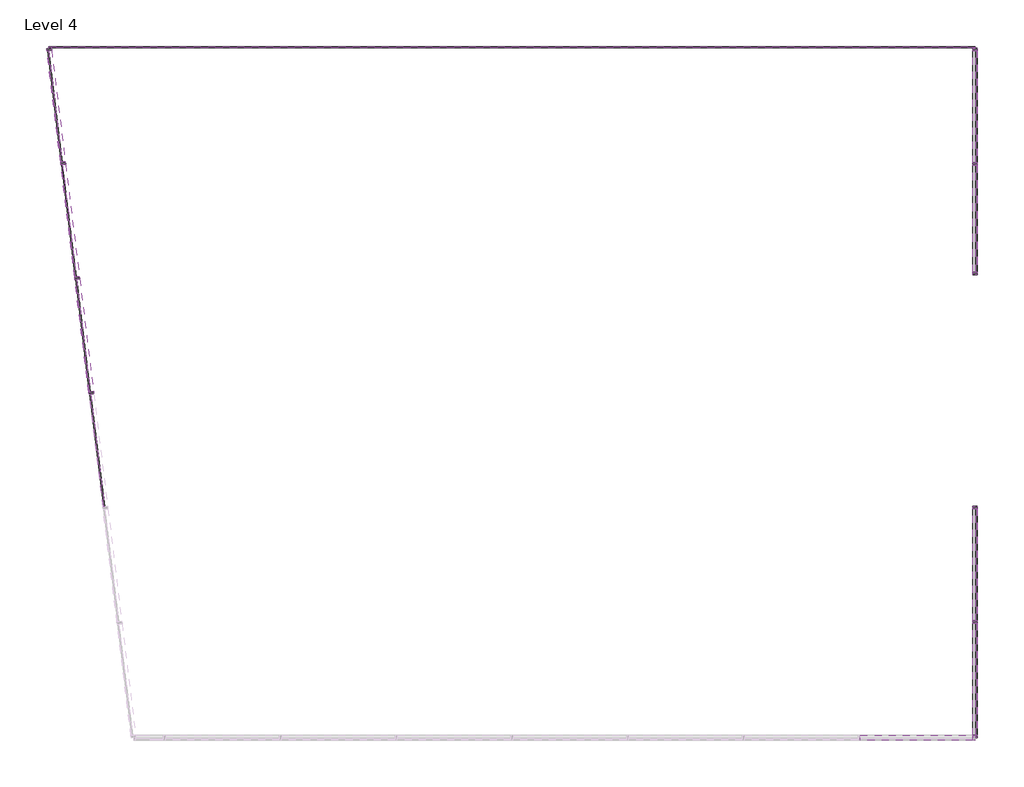
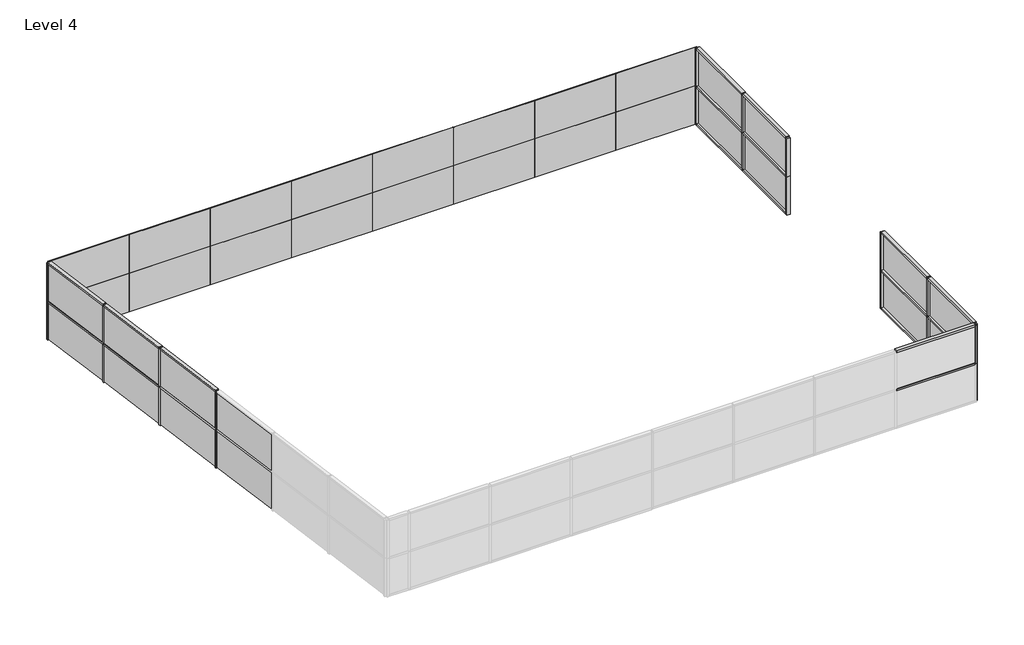
# One storey, part 2 of 2: 41 members, 32 plates.
"""IFC4 building model written with IfcOpenShell, lengths in millimetres."""

from ifc_helpers import new_model, si_unit, origin, place, context, project, spatial, transform, mapped, element, save
from components import member_71c27fd2, member_19d0a4ec, member_8cef0660, member_82905deb, member_4491d118, member_1b94d493, member_46bdb8c2, system_panel_glazed_1e57f9bb, system_panel_glazed_37f15d2e, system_panel_glazed_e46d4b42, system_panel_glazed_2a6c68b7, system_panel_glazed_7fb1fc2b, system_panel_glazed_d483336f

model = new_model("IFC4")

# Units and contexts
model_context = context("Model", 3, world=origin())
ifc_project = project(units=[si_unit("LENGTHUNIT", "METRE", prefix="MILLI")], contexts=[model_context])

# Site, building, storey
site = spatial("IfcSite", under=ifc_project)
building = spatial("IfcBuilding", under=site)
storey = spatial("IfcBuildingStorey", under=building, Name="Level 4", Elevation=9144.0)

# Members
placement = place(None, origin())
member_shape = member_71c27fd2(model_context)
element("IfcMember", 1, ObjectType="Rectangular Mullion : 2.5\" x 5\" rectangular", at=placement, inside=storey, context=model_context, shape_type="MappedRepresentation", body=[
    mapped(member_shape, transform((13902.5156363, -6915.6363705, 9144.0), x_axis=(0.0, 0.0, -1.0), y_axis=(1.0, 0.0, 0.0), z_axis=(0.0, -1.0, 0.0))),
])
element("IfcMember", 2, ObjectType="Rectangular Mullion : 2.5\" x 5\" rectangular", at=placement, inside=storey, context=model_context, shape_type="MappedRepresentation", body=[
    mapped(member_shape, transform((13902.5156363, -3899.3863708, 9144.0), x_axis=(0.0, 0.0, -1.0), y_axis=(1.0, 0.0, 0.0), z_axis=(0.0, -1.0, 0.0))),
])
element("IfcMember", 3, ObjectType="Rectangular Mullion : 2.5\" x 5\" rectangular", at=placement, inside=storey, context=model_context, shape_type="MappedRepresentation", body=[
    mapped(member_shape, transform((13902.5156363, 8156.2976505, 9144.0), x_axis=(0.0, 0.0, -1.0), y_axis=(1.0, 0.0, 0.0), z_axis=(0.0, -1.0, 0.0))),
])
member_2_shape = member_19d0a4ec(model_context)
element("IfcMember", 4, ObjectType="Rectangular Mullion : 2.5\" x 5\" rectangular", at=placement, inside=storey, context=model_context, shape_type="MappedRepresentation", body=[
    mapped(member_2_shape, transform((13839.0156363, -6979.1363705, 10668.0), x_axis=(0.0, 0.0, 1.0), y_axis=(0.0, -1.0, 0.0), z_axis=(1.0, 0.0, 0.0))),
])
element("IfcMember", 5, ObjectType="Rectangular Mullion : 2.5\" x 5\" rectangular", at=placement, inside=storey, context=model_context, shape_type="MappedRepresentation", body=[
    mapped(member_2_shape, transform((13839.0156363, -6979.1363705, 12192.0), x_axis=(0.0, 0.0, 1.0), y_axis=(0.0, -1.0, 0.0), z_axis=(1.0, 0.0, 0.0))),
])
element("IfcMember", 6, ObjectType="Rectangular Mullion : 2.5\" x 5\" rectangular", at=placement, inside=storey, context=model_context, shape_type="MappedRepresentation", body=[
    mapped(member_2_shape, transform((-10113.8959567, 8178.7803212, 10668.0), x_axis=(0.0, 0.0, 1.0), y_axis=(-0.9925461516413222, -0.12186934340514609, 0.0), z_axis=(0.12186934340514609, -0.9925461516413222, 0.0))),
])
element("IfcMember", 7, ObjectType="Rectangular Mullion : 2.5\" x 5\" rectangular", at=placement, inside=storey, context=model_context, shape_type="MappedRepresentation", body=[
    mapped(member_2_shape, transform((-10113.8959567, 8178.7803212, 12192.0), x_axis=(0.0, 0.0, 1.0), y_axis=(-0.9925461516413222, -0.12186934340514617, 0.0), z_axis=(0.12186934340514617, -0.9925461516413222, 0.0))),
])
element("IfcMember", 8, ObjectType="Rectangular Mullion : 2.5\" x 5\" rectangular", at=placement, inside=storey, context=model_context, shape_type="MappedRepresentation", body=[
    mapped(member_2_shape, transform((13902.5156363, -946.6363705, 10668.0), x_axis=(0.0, 0.0, 1.0), y_axis=(1.0, 0.0, 0.0), z_axis=(0.0, 1.0, 0.0))),
])
element("IfcMember", 9, ObjectType="Rectangular Mullion : 2.5\" x 5\" rectangular", at=placement, inside=storey, context=model_context, shape_type="MappedRepresentation", body=[
    mapped(member_2_shape, transform((13902.5156363, -3962.8863708, 10668.0), x_axis=(0.0, 0.0, 1.0), y_axis=(1.0, 0.0, 0.0), z_axis=(0.0, 1.0, 0.0))),
])
element("IfcMember", 10, ObjectType="Rectangular Mullion : 2.5\" x 5\" rectangular", at=placement, inside=storey, context=model_context, shape_type="MappedRepresentation", body=[
    mapped(member_2_shape, transform((13902.5156363, -946.6363705, 12192.0), x_axis=(0.0, 0.0, 1.0), y_axis=(1.0, 0.0, 0.0), z_axis=(0.0, 1.0, 0.0))),
])
element("IfcMember", 11, ObjectType="Rectangular Mullion : 2.5\" x 5\" rectangular", at=placement, inside=storey, context=model_context, shape_type="MappedRepresentation", body=[
    mapped(member_2_shape, transform((13902.5156363, -3962.8863708, 12192.0), x_axis=(0.0, 0.0, 1.0), y_axis=(1.0, 0.0, 0.0), z_axis=(0.0, 1.0, 0.0))),
])
element("IfcMember", 12, ObjectType="Rectangular Mullion : 2.5\" x 5\" rectangular", at=placement, inside=storey, context=model_context, shape_type="MappedRepresentation", body=[
    mapped(member_2_shape, transform((13902.5156363, 11109.0476508, 10668.0), x_axis=(0.0, 0.0, 1.0), y_axis=(1.0, 0.0, 0.0), z_axis=(0.0, 1.0, 0.0))),
])
element("IfcMember", 13, ObjectType="Rectangular Mullion : 2.5\" x 5\" rectangular", at=placement, inside=storey, context=model_context, shape_type="MappedRepresentation", body=[
    mapped(member_2_shape, transform((13902.5156363, 11109.0476508, 12192.0), x_axis=(0.0, 0.0, 1.0), y_axis=(1.0, 0.0, 0.0), z_axis=(0.0, 1.0, 0.0))),
])
member_3_shape = member_8cef0660(model_context)
element("IfcMember", 14, ObjectType="Rectangular Mullion : 2.5\" x 5\" rectangular", at=placement, inside=storey, context=model_context, shape_type="MappedRepresentation", body=[
    mapped(member_3_shape, transform((-9370.9804393, 2128.2189808, 10668.0), x_axis=(0.0, 0.0, 1.0), y_axis=(-0.9925461516413223, -0.12186934340514563, 0.0), z_axis=(0.12186934340514562, -0.9925461516413222, 0.0))),
])
element("IfcMember", 15, ObjectType="Rectangular Mullion : 2.5\" x 5\" rectangular", at=placement, inside=storey, context=model_context, shape_type="MappedRepresentation", body=[
    mapped(member_3_shape, transform((-9742.438198, 5153.499651, 10668.0), x_axis=(0.0, 0.0, 1.0), y_axis=(-0.9925461516413222, -0.12186934340514602, 0.0), z_axis=(0.12186934340514602, -0.9925461516413222, 0.0))),
])
element("IfcMember", 16, ObjectType="Rectangular Mullion : 2.5\" x 5\" rectangular", at=placement, inside=storey, context=model_context, shape_type="MappedRepresentation", body=[
    mapped(member_3_shape, transform((-9370.9804393, 2128.2189808, 12192.0), x_axis=(0.0, 0.0, 1.0), y_axis=(-0.9925461516413222, -0.12186934340514596, 0.0), z_axis=(0.12186934340514596, -0.9925461516413222, 0.0))),
])
element("IfcMember", 17, ObjectType="Rectangular Mullion : 2.5\" x 5\" rectangular", at=placement, inside=storey, context=model_context, shape_type="MappedRepresentation", body=[
    mapped(member_3_shape, transform((-9742.438198, 5153.499651, 12192.0), x_axis=(0.0, 0.0, 1.0), y_axis=(-0.9925461516413222, -0.12186934340514566, 0.0), z_axis=(0.12186934340514566, -0.9925461516413222, 0.0))),
])
member_4_shape = member_82905deb(model_context)
element("IfcMember", 18, ObjectType="Rectangular Mullion : 2.5\" x 5\" rectangular", at=placement, inside=storey, context=model_context, shape_type="MappedRepresentation", body=[
    mapped(member_4_shape, transform((13902.5156363, -3931.1363708, 10668.0), x_axis=(0.0, -1.0, 0.0), y_axis=(1.0, 0.0, 0.0), z_axis=(0.0, 0.0, 1.0))),
])
element("IfcMember", 19, ObjectType="Rectangular Mullion : 2.5\" x 5\" rectangular", at=placement, inside=storey, context=model_context, shape_type="MappedRepresentation", body=[
    mapped(member_4_shape, transform((13902.5156363, 8124.5476505, 10668.0), x_axis=(0.0, -1.0, 0.0), y_axis=(1.0, 0.0, 0.0), z_axis=(0.0, 0.0, 1.0))),
])
element("IfcMember", 20, ObjectType="Rectangular Mullion : 2.5\" x 5\" rectangular", at=placement, inside=storey, context=model_context, shape_type="MappedRepresentation", body=[
    mapped(member_4_shape, transform((-9367.1110876, 2096.7056405, 10668.0), x_axis=(-0.1218693434051459, 0.9925461516413222, 0.0), y_axis=(-0.9925461516413222, -0.1218693434051459, 0.0), z_axis=(0.0, 0.0, 1.0))),
])
element("IfcMember", 21, ObjectType="Rectangular Mullion : 2.5\" x 5\" rectangular", at=placement, inside=storey, context=model_context, shape_type="MappedRepresentation", body=[
    mapped(member_4_shape, transform((-9367.1110876, 2096.7056405, 12192.0), x_axis=(-0.1218693434051459, 0.9925461516413222, 0.0), y_axis=(-0.9925461516413222, -0.1218693434051459, 0.0), z_axis=(0.0, 0.0, 1.0))),
])
element("IfcMember", 22, ObjectType="Rectangular Mullion : 2.5\" x 5\" rectangular", at=placement, inside=storey, context=model_context, shape_type="MappedRepresentation", body=[
    mapped(member_4_shape, transform((-9738.5688463, 5121.9863107, 10668.0), x_axis=(-0.1218693434051459, 0.9925461516413222, 0.0), y_axis=(-0.9925461516413222, -0.1218693434051459, 0.0), z_axis=(0.0, 0.0, 1.0))),
])
element("IfcMember", 23, ObjectType="Rectangular Mullion : 2.5\" x 5\" rectangular", at=placement, inside=storey, context=model_context, shape_type="MappedRepresentation", body=[
    mapped(member_4_shape, transform((-9738.5688463, 5121.9863107, 12192.0), x_axis=(-0.1218693434051459, 0.9925461516413222, 0.0), y_axis=(-0.9925461516413222, -0.1218693434051459, 0.0), z_axis=(0.0, 0.0, 1.0))),
])
element("IfcMember", 24, ObjectType="Rectangular Mullion : 2.5\" x 5\" rectangular", at=placement, inside=storey, context=model_context, shape_type="MappedRepresentation", body=[
    mapped(member_4_shape, transform((-10110.026605, 8147.2669809, 10668.0), x_axis=(-0.1218693434051459, 0.9925461516413222, 0.0), y_axis=(-0.9925461516413222, -0.1218693434051459, 0.0), z_axis=(0.0, 0.0, 1.0))),
])
element("IfcMember", 25, ObjectType="Rectangular Mullion : 2.5\" x 5\" rectangular", at=placement, inside=storey, context=model_context, shape_type="MappedRepresentation", body=[
    mapped(member_4_shape, transform((-10110.026605, 8147.2669809, 12192.0), x_axis=(-0.1218693434051459, 0.9925461516413222, 0.0), y_axis=(-0.9925461516413222, -0.1218693434051459, 0.0), z_axis=(0.0, 0.0, 1.0))),
])
element("IfcMember", 26, ObjectType="Rectangular Mullion : 2.5\" x 5\" rectangular", at=placement, inside=storey, context=model_context, shape_type="MappedRepresentation", body=[
    mapped(member_4_shape, transform((13902.5156363, -3931.1363708, 12192.0), x_axis=(0.0, -1.0, 0.0), y_axis=(1.0, 0.0, 0.0), z_axis=(0.0, 0.0, 1.0))),
])
element("IfcMember", 27, ObjectType="Rectangular Mullion : 2.5\" x 5\" rectangular", at=placement, inside=storey, context=model_context, shape_type="MappedRepresentation", body=[
    mapped(member_4_shape, transform((13902.5156363, 8124.5476505, 12192.0), x_axis=(0.0, -1.0, 0.0), y_axis=(1.0, 0.0, 0.0), z_axis=(0.0, 0.0, 1.0))),
])
member_5_shape = member_4491d118(model_context)
element("IfcMember", 28, ObjectType="Rectangular Mullion : 2.5\" x 5\" rectangular", at=placement, inside=storey, context=model_context, shape_type="MappedRepresentation", body=[
    mapped(member_5_shape, transform((13902.5156363, -883.1363705, 9144.0), x_axis=(0.0, 1.0, 0.0), y_axis=(1.0, 0.0, 0.0), z_axis=(0.0, 0.0, -1.0))),
])
element("IfcMember", 29, ObjectType="Rectangular Mullion : 2.5\" x 5\" rectangular", at=placement, inside=storey, context=model_context, shape_type="MappedRepresentation", body=[
    mapped(member_5_shape, transform((13902.5156363, 11172.5476508, 9144.0), x_axis=(0.0, 1.0, 0.0), y_axis=(1.0, 0.0, 0.0), z_axis=(0.0, 0.0, -1.0))),
])
element("IfcMember", 30, ObjectType="Rectangular Mullion : 2.5\" x 5\" rectangular", at=placement, inside=storey, context=model_context, shape_type="MappedRepresentation", body=[
    mapped(member_5_shape, transform((13902.5156363, -6979.1363705, 10668.0), x_axis=(1.0, 0.0, 0.0), y_axis=(0.0, -1.0, 0.0), z_axis=(0.0, 0.0, -1.0))),
])
element("IfcMember", 31, ObjectType="Rectangular Mullion : 2.5\" x 5\" rectangular", at=placement, inside=storey, context=model_context, shape_type="MappedRepresentation", body=[
    mapped(member_5_shape, transform((13902.5156363, -883.1363705, 10668.0), x_axis=(0.0, 1.0, 0.0), y_axis=(1.0, 0.0, 0.0), z_axis=(0.0, 0.0, -1.0))),
])
element("IfcMember", 32, ObjectType="Rectangular Mullion : 2.5\" x 5\" rectangular", at=placement, inside=storey, context=model_context, shape_type="MappedRepresentation", body=[
    mapped(member_5_shape, transform((13902.5156363, 11172.5476508, 10668.0), x_axis=(0.0, 1.0, 0.0), y_axis=(1.0, 0.0, 0.0), z_axis=(0.0, 0.0, -1.0))),
])
element("IfcMember", 33, ObjectType="Rectangular Mullion : 2.5\" x 5\" rectangular", at=placement, inside=storey, context=model_context, shape_type="MappedRepresentation", body=[
    mapped(member_5_shape, transform((13902.5156363, -6979.1363705, 10668.0), x_axis=(0.0, -1.0, 0.0), y_axis=(1.0, 0.0, 0.0), z_axis=(0.0, 0.0, 1.0))),
])
element("IfcMember", 34, ObjectType="Rectangular Mullion : 2.5\" x 5\" rectangular", at=placement, inside=storey, context=model_context, shape_type="MappedRepresentation", body=[
    mapped(member_5_shape, transform((13902.5156363, 5212.8636295, 10668.0), x_axis=(0.0, -1.0, 0.0), y_axis=(1.0, 0.0, 0.0), z_axis=(0.0, 0.0, 1.0))),
])
element("IfcMember", 35, ObjectType="Rectangular Mullion : 2.5\" x 5\" rectangular", at=placement, inside=storey, context=model_context, shape_type="MappedRepresentation", body=[
    mapped(member_5_shape, transform((-10481.4843637, 11172.5476508, 10668.0), x_axis=(-0.1218693434051459, 0.9925461516413222, 0.0), y_axis=(-0.9925461516413222, -0.1218693434051459, 0.0), z_axis=(0.0, 0.0, 1.0))),
])
element("IfcMember", 36, ObjectType="Rectangular Mullion : 2.5\" x 5\" rectangular", at=placement, inside=storey, context=model_context, shape_type="MappedRepresentation", body=[
    mapped(member_5_shape, transform((-10481.4843637, 11172.5476508, 12192.0), x_axis=(-0.1218693434051459, 0.9925461516413222, 0.0), y_axis=(-0.9925461516413222, -0.1218693434051459, 0.0), z_axis=(0.0, 0.0, 1.0))),
])
element("IfcMember", 37, ObjectType="Rectangular Mullion : 2.5\" x 5\" rectangular", at=placement, inside=storey, context=model_context, shape_type="MappedRepresentation", body=[
    mapped(member_5_shape, transform((13902.5156363, -6979.1363705, 12192.0), x_axis=(0.0, -1.0, 0.0), y_axis=(1.0, 0.0, 0.0), z_axis=(0.0, 0.0, 1.0))),
])
element("IfcMember", 38, ObjectType="Rectangular Mullion : 2.5\" x 5\" rectangular", at=placement, inside=storey, context=model_context, shape_type="MappedRepresentation", body=[
    mapped(member_5_shape, transform((13902.5156363, 5212.8636295, 12192.0), x_axis=(0.0, -1.0, 0.0), y_axis=(1.0, 0.0, 0.0), z_axis=(0.0, 0.0, 1.0))),
])
member_6_shape = member_1b94d493(model_context)
element("IfcMember", 39, ObjectType="Rectangular Mullion : 2.5\" x 5\" rectangular", at=placement, inside=storey, context=model_context, shape_type="MappedRepresentation", body=[
    mapped(member_6_shape, transform((13902.5156363, 5276.3636295, 9144.0), x_axis=(0.0, 0.0, -1.0), y_axis=(1.0, 0.0, 0.0), z_axis=(0.0, -1.0, 0.0))),
])
member_7_shape = member_46bdb8c2(model_context)
element("IfcMember", 40, ObjectType="Rectangular Mullion : 2.5\" x 5\" rectangular", at=placement, inside=storey, context=model_context, shape_type="MappedRepresentation", body=[
    mapped(member_7_shape, transform((13902.5156363, 8092.7976505, 10668.0), x_axis=(0.0, 0.0, 1.0), y_axis=(1.0, 0.0, 0.0), z_axis=(0.0, 1.0, 0.0))),
])
element("IfcMember", 41, ObjectType="Rectangular Mullion : 2.5\" x 5\" rectangular", at=placement, inside=storey, context=model_context, shape_type="MappedRepresentation", body=[
    mapped(member_7_shape, transform((13902.5156363, 8092.7976505, 12192.0), x_axis=(0.0, 0.0, 1.0), y_axis=(1.0, 0.0, 0.0), z_axis=(0.0, 1.0, 0.0))),
])

# Plates
system_panel_glazed_shape = system_panel_glazed_1e57f9bb(model_context)
element("IfcPlate", 42, ObjectType="System Panel : Glazed", at=placement, inside=storey, context=model_context, shape_type="MappedRepresentation", body=[
    mapped(system_panel_glazed_shape, transform((-8957.4843636, 11172.5476508, 9144.0), x_axis=(1.0, 0.0, 0.0), y_axis=(0.0, 1.0, 0.0), z_axis=(0.0, 0.0, 1.0))),
])
element("IfcPlate", 43, ObjectType="System Panel : Glazed", at=placement, inside=storey, context=model_context, shape_type="MappedRepresentation", body=[
    mapped(system_panel_glazed_shape, transform((-5909.4843634, 11172.5476508, 9144.0), x_axis=(1.0, 0.0, 0.0), y_axis=(0.0, 1.0, 0.0), z_axis=(0.0, 0.0, 1.0))),
])
element("IfcPlate", 44, ObjectType="System Panel : Glazed", at=placement, inside=storey, context=model_context, shape_type="MappedRepresentation", body=[
    mapped(system_panel_glazed_shape, transform((-2861.4843634, 11172.5476508, 9144.0), x_axis=(1.0, 0.0, 0.0), y_axis=(0.0, 1.0, 0.0), z_axis=(0.0, 0.0, 1.0))),
])
element("IfcPlate", 45, ObjectType="System Panel : Glazed", at=placement, inside=storey, context=model_context, shape_type="MappedRepresentation", body=[
    mapped(system_panel_glazed_shape, transform((186.5156366, 11172.5476508, 9144.0), x_axis=(1.0, 0.0, 0.0), y_axis=(0.0, 1.0, 0.0), z_axis=(0.0, 0.0, 1.0))),
])
element("IfcPlate", 46, ObjectType="System Panel : Glazed", at=placement, inside=storey, context=model_context, shape_type="MappedRepresentation", body=[
    mapped(system_panel_glazed_shape, transform((3234.5156366, 11172.5476508, 9144.0), x_axis=(1.0, 0.0, 0.0), y_axis=(0.0, 1.0, 0.0), z_axis=(0.0, 0.0, 1.0))),
])
element("IfcPlate", 47, ObjectType="System Panel : Glazed", at=placement, inside=storey, context=model_context, shape_type="MappedRepresentation", body=[
    mapped(system_panel_glazed_shape, transform((6282.5156366, 11172.5476508, 9144.0), x_axis=(1.0, 0.0, 0.0), y_axis=(0.0, 1.0, 0.0), z_axis=(0.0, 0.0, 1.0))),
])
element("IfcPlate", 48, ObjectType="System Panel : Glazed", at=placement, inside=storey, context=model_context, shape_type="MappedRepresentation", body=[
    mapped(system_panel_glazed_shape, transform((9330.5156366, 11172.5476508, 9144.0), x_axis=(1.0, 0.0, 0.0), y_axis=(0.0, 1.0, 0.0), z_axis=(0.0, 0.0, 1.0))),
])
element("IfcPlate", 49, ObjectType="System Panel : Glazed", at=placement, inside=storey, context=model_context, shape_type="MappedRepresentation", body=[
    mapped(system_panel_glazed_shape, transform((12378.5156364, 11172.5476508, 9144.0), x_axis=(1.0, 0.0, 0.0), y_axis=(0.0, 1.0, 0.0), z_axis=(0.0, 0.0, 1.0))),
])
element("IfcPlate", 50, ObjectType="System Panel : Glazed", at=placement, inside=storey, context=model_context, shape_type="MappedRepresentation", body=[
    mapped(system_panel_glazed_shape, transform((-8957.4843636, 11172.5476508, 10668.0), x_axis=(1.0, 0.0, 0.0), y_axis=(0.0, 1.0, 0.0), z_axis=(0.0, 0.0, 1.0))),
])
element("IfcPlate", 51, ObjectType="System Panel : Glazed", at=placement, inside=storey, context=model_context, shape_type="MappedRepresentation", body=[
    mapped(system_panel_glazed_shape, transform((-5909.4843634, 11172.5476508, 10668.0), x_axis=(1.0, 0.0, 0.0), y_axis=(0.0, 1.0, 0.0), z_axis=(0.0, 0.0, 1.0))),
])
element("IfcPlate", 52, ObjectType="System Panel : Glazed", at=placement, inside=storey, context=model_context, shape_type="MappedRepresentation", body=[
    mapped(system_panel_glazed_shape, transform((-2861.4843634, 11172.5476508, 10668.0), x_axis=(1.0, 0.0, 0.0), y_axis=(0.0, 1.0, 0.0), z_axis=(0.0, 0.0, 1.0))),
])
element("IfcPlate", 53, ObjectType="System Panel : Glazed", at=placement, inside=storey, context=model_context, shape_type="MappedRepresentation", body=[
    mapped(system_panel_glazed_shape, transform((186.5156366, 11172.5476508, 10668.0), x_axis=(1.0, 0.0, 0.0), y_axis=(0.0, 1.0, 0.0), z_axis=(0.0, 0.0, 1.0))),
])
element("IfcPlate", 54, ObjectType="System Panel : Glazed", at=placement, inside=storey, context=model_context, shape_type="MappedRepresentation", body=[
    mapped(system_panel_glazed_shape, transform((3234.5156366, 11172.5476508, 10668.0), x_axis=(1.0, 0.0, 0.0), y_axis=(0.0, 1.0, 0.0), z_axis=(0.0, 0.0, 1.0))),
])
element("IfcPlate", 55, ObjectType="System Panel : Glazed", at=placement, inside=storey, context=model_context, shape_type="MappedRepresentation", body=[
    mapped(system_panel_glazed_shape, transform((6282.5156366, 11172.5476508, 10668.0), x_axis=(1.0, 0.0, 0.0), y_axis=(0.0, 1.0, 0.0), z_axis=(0.0, 0.0, 1.0))),
])
element("IfcPlate", 56, ObjectType="System Panel : Glazed", at=placement, inside=storey, context=model_context, shape_type="MappedRepresentation", body=[
    mapped(system_panel_glazed_shape, transform((9330.5156366, 11172.5476508, 10668.0), x_axis=(1.0, 0.0, 0.0), y_axis=(0.0, 1.0, 0.0), z_axis=(0.0, 0.0, 1.0))),
])
element("IfcPlate", 57, ObjectType="System Panel : Glazed", at=placement, inside=storey, context=model_context, shape_type="MappedRepresentation", body=[
    mapped(system_panel_glazed_shape, transform((12378.5156364, 11172.5476508, 10668.0), x_axis=(1.0, 0.0, 0.0), y_axis=(0.0, 1.0, 0.0), z_axis=(0.0, 0.0, 1.0))),
])
system_panel_glazed_2_shape = system_panel_glazed_37f15d2e(model_context)
element("IfcPlate", 58, ObjectType="System Panel : Glazed", at=placement, inside=storey, context=model_context, shape_type="MappedRepresentation", body=[
    mapped(system_panel_glazed_2_shape, transform((13902.5156363, -2423.0113706, 9207.5), x_axis=(0.0, -1.0, 0.0), y_axis=(1.0, 0.0, 0.0), z_axis=(0.0, 0.0, 1.0))),
])
element("IfcPlate", 59, ObjectType="System Panel : Glazed", at=placement, inside=storey, context=model_context, shape_type="MappedRepresentation", body=[
    mapped(system_panel_glazed_2_shape, transform((13902.5156363, 9632.6726506, 9207.5), x_axis=(0.0, -1.0, 0.0), y_axis=(1.0, 0.0, 0.0), z_axis=(0.0, 0.0, 1.0))),
])
element("IfcPlate", 60, ObjectType="System Panel : Glazed", at=placement, inside=storey, context=model_context, shape_type="MappedRepresentation", body=[
    mapped(system_panel_glazed_2_shape, transform((13902.5156363, -5439.2613706, 9207.5), x_axis=(0.0, -1.0, 0.0), y_axis=(1.0, 0.0, 0.0), z_axis=(0.0, 0.0, 1.0))),
])
system_panel_glazed_3_shape = system_panel_glazed_e46d4b42(model_context)
element("IfcPlate", 61, ObjectType="System Panel : Glazed", at=placement, inside=storey, context=model_context, shape_type="MappedRepresentation", body=[
    mapped(system_panel_glazed_3_shape, transform((-10293.8208085, 9644.1506457, 9175.75), x_axis=(-0.1218693434051459, 0.9925461516413222, 0.0), y_axis=(-0.9925461516413222, -0.1218693434051459, 0.0), z_axis=(0.0, 0.0, 1.0))),
])
element("IfcPlate", 62, ObjectType="System Panel : Glazed", at=placement, inside=storey, context=model_context, shape_type="MappedRepresentation", body=[
    mapped(system_panel_glazed_3_shape, transform((-10293.8208085, 9644.1506457, 10699.75), x_axis=(-0.1218693434051459, 0.9925461516413222, 0.0), y_axis=(-0.9925461516413222, -0.1218693434051459, 0.0), z_axis=(0.0, 0.0, 1.0))),
])
element("IfcPlate", 63, ObjectType="System Panel : Glazed", at=placement, inside=storey, context=model_context, shape_type="MappedRepresentation", body=[
    mapped(system_panel_glazed_3_shape, transform((13902.5156363, -2423.0113706, 10699.75), x_axis=(0.0, -1.0, 0.0), y_axis=(1.0, 0.0, 0.0), z_axis=(0.0, 0.0, 1.0))),
])
element("IfcPlate", 64, ObjectType="System Panel : Glazed", at=placement, inside=storey, context=model_context, shape_type="MappedRepresentation", body=[
    mapped(system_panel_glazed_3_shape, transform((13902.5156363, -5439.2613706, 10699.75), x_axis=(0.0, -1.0, 0.0), y_axis=(1.0, 0.0, 0.0), z_axis=(0.0, 0.0, 1.0))),
])
element("IfcPlate", 65, ObjectType="System Panel : Glazed", at=placement, inside=storey, context=model_context, shape_type="MappedRepresentation", body=[
    mapped(system_panel_glazed_3_shape, transform((13902.5156363, 9632.6726506, 10699.75), x_axis=(0.0, -1.0, 0.0), y_axis=(1.0, 0.0, 0.0), z_axis=(0.0, 0.0, 1.0))),
])
system_panel_glazed_4_shape = system_panel_glazed_2a6c68b7(model_context)
element("IfcPlate", 66, ObjectType="System Panel : Glazed", at=placement, inside=storey, context=model_context, shape_type="MappedRepresentation", body=[
    mapped(system_panel_glazed_4_shape, transform((-9181.3822083, 584.0653054, 9175.75), x_axis=(-0.1218693434051459, 0.9925461516413222, 0.0), y_axis=(-0.9925461516413222, -0.1218693434051459, 0.0), z_axis=(0.0, 0.0, 1.0))),
])
element("IfcPlate", 67, ObjectType="System Panel : Glazed", at=placement, inside=storey, context=model_context, shape_type="MappedRepresentation", body=[
    mapped(system_panel_glazed_4_shape, transform((-9552.839967, 3609.3459756, 9175.75), x_axis=(-0.1218693434051459, 0.9925461516413222, 0.0), y_axis=(-0.9925461516413222, -0.1218693434051459, 0.0), z_axis=(0.0, 0.0, 1.0))),
])
element("IfcPlate", 68, ObjectType="System Panel : Glazed", at=placement, inside=storey, context=model_context, shape_type="MappedRepresentation", body=[
    mapped(system_panel_glazed_4_shape, transform((-9924.2977257, 6634.6266458, 9175.75), x_axis=(-0.1218693434051459, 0.9925461516413222, 0.0), y_axis=(-0.9925461516413222, -0.1218693434051459, 0.0), z_axis=(0.0, 0.0, 1.0))),
])
element("IfcPlate", 69, ObjectType="System Panel : Glazed", at=placement, inside=storey, context=model_context, shape_type="MappedRepresentation", body=[
    mapped(system_panel_glazed_4_shape, transform((-9181.3822083, 584.0653054, 10699.75), x_axis=(-0.1218693434051459, 0.9925461516413222, 0.0), y_axis=(-0.9925461516413222, -0.1218693434051459, 0.0), z_axis=(0.0, 0.0, 1.0))),
])
element("IfcPlate", 70, ObjectType="System Panel : Glazed", at=placement, inside=storey, context=model_context, shape_type="MappedRepresentation", body=[
    mapped(system_panel_glazed_4_shape, transform((-9552.839967, 3609.3459756, 10699.75), x_axis=(-0.1218693434051459, 0.9925461516413222, 0.0), y_axis=(-0.9925461516413222, -0.1218693434051459, 0.0), z_axis=(0.0, 0.0, 1.0))),
])
element("IfcPlate", 71, ObjectType="System Panel : Glazed", at=placement, inside=storey, context=model_context, shape_type="MappedRepresentation", body=[
    mapped(system_panel_glazed_4_shape, transform((-9924.2977257, 6634.6266458, 10699.75), x_axis=(-0.1218693434051459, 0.9925461516413222, 0.0), y_axis=(-0.9925461516413222, -0.1218693434051459, 0.0), z_axis=(0.0, 0.0, 1.0))),
])
system_panel_glazed_5_shape = system_panel_glazed_7fb1fc2b(model_context)
element("IfcPlate", 72, ObjectType="System Panel : Glazed", at=placement, inside=storey, context=model_context, shape_type="MappedRepresentation", body=[
    mapped(system_panel_glazed_5_shape, transform((13902.5156363, 6684.58064, 9207.5), x_axis=(0.0, -1.0, 0.0), y_axis=(1.0, 0.0, 0.0), z_axis=(0.0, 0.0, 1.0))),
])
system_panel_glazed_6_shape = system_panel_glazed_d483336f(model_context)
element("IfcPlate", 73, ObjectType="System Panel : Glazed", at=placement, inside=storey, context=model_context, shape_type="MappedRepresentation", body=[
    mapped(system_panel_glazed_6_shape, transform((13902.5156363, 6684.58064, 10699.75), x_axis=(0.0, -1.0, 0.0), y_axis=(1.0, 0.0, 0.0), z_axis=(0.0, 0.0, 1.0))),
])

save(model, "model.ifc")

# Revit data of these elements
# Type "Rectangular Mullion : 2.5\" x 5\" rectangular"
#   built-in parameter 1007304 = 0.416667 (stored number, unit not read)
#   built-in parameter 1007301 = 0.104167 (stored number, unit not read)
#   built-in parameter 1007300 = 0.104167 (stored number, unit not read)
# Type "System Panel : Glazed"
#   Construction Type Id = "GSP4R"
#   Analytic Construction = "1/8 in Pilkington single glazing"
#   Visual Light Transmittance = 0.9
#   Solar Heat Gain Coefficient = 0.86
#   Heat Transfer Coefficient (U) = 1.18115 BTU/(h·ft²·°F)
#   Define Thermal Properties by = 1
# Elements 1, 2, 3, 4, 5, 6, 7, 8, 9, 10, 11, 12, 13, 14, 15, 16, 17, 18, 19, 20, 21, 22, 23, 24, 25, 26, 27, 28, 29, 30, 31, 32, 33, 34, 35, 36, 37, 38, 39, 40, 41 (IfcMember, "Rectangular Mullion : 2.5\" x 5\" rectangular")
#   Phase Created = New Construction
#   Materials on its faces: "Aluminum"
# Elements 42, 43, 44, 45, 46, 47, 48, 49, 50, 51, 52, 53, 54, 55, 56, 57, 58, 59, 60, 61, 62, 63, 64, 65, 66, 67, 68, 69, 70, 71, 72, 73 (IfcPlate, "System Panel : Glazed")
#   Phase Created = New Construction
#   Materials on its faces: "Glass"
# Materials
#   "Aluminum": class "Metal", colour RGB 247 247 247, transparency 0, Description = "Aluminum 6061", Cost = 0
#   "Glass": class "Glass", colour RGB 0 128 192, transparency 0.75, Description = "Soda Lime Glass", Cost = 0
